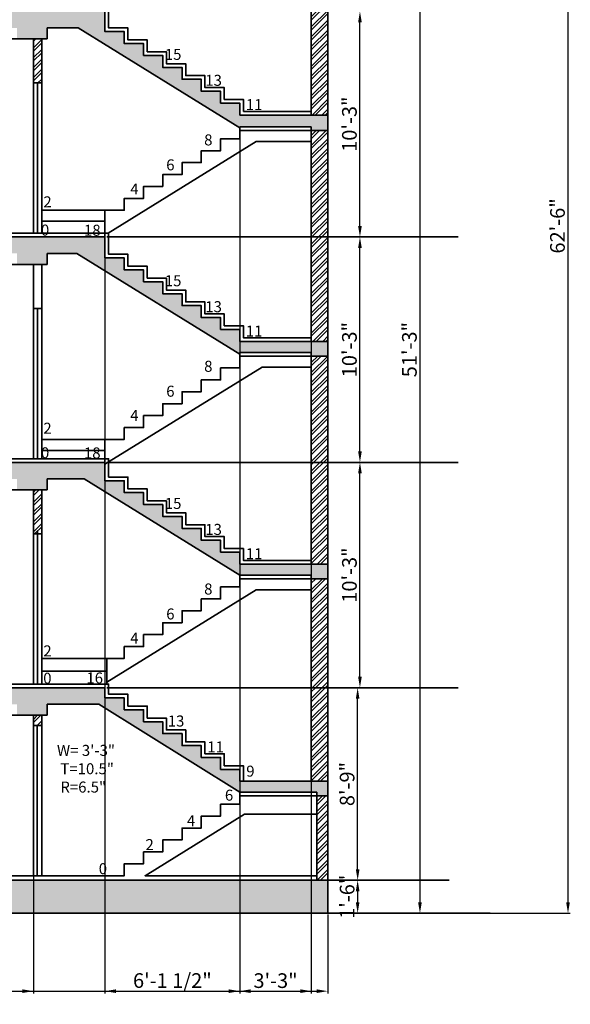
# Model space of a CAD drawing. Units: millimetres. Extents: x 1706 to 5913, y 156 to 1716.
# Tile 19 of 26: x 4807 to 5108, y 156 to 693. Entities that reach past the tile are written whole.
import ezdxf

# ---------------------------------------------------------------- set-up
doc = ezdxf.new("R2010")
doc.units = ezdxf.units.MM
for name, color, linetype, lineweight in [('A-ANNO-DIMS', 2, 'Continuous', 18), ('A-ANNO-TEXT', 7, 'Continuous', 18), ('A-SECT', 7, 'Continuous', 35), ('A-SECT-PATT', 8, 'Continuous', 13)]:
    doc.layers.add(name, color=color, linetype=linetype, lineweight=lineweight)
doc.styles.get("Standard").update_dxf_attribs({"font": 'arial.ttf'})
doc.dimstyles.new('ISO-25', dxfattribs={"dimtxt": 8, "dimasz": 6, "dimexe": 1.25, "dimexo": 0.625, "dimtad": 1, "dimdec": 0, "dimlunit": 3, "dimtxsty": 'Standard', "dimcen": 2.5, "dimadec": 0, "dimazin": 0, "dimtfac": 1, "dimtdec": 0, "dimtmove": 0, "dimatfit": 3, "dimfxl": 1, "dimarcsym": 0})
pattern_1 = [(45, (229.4607, 1496.8062), (-2.6940768, 2.6940768), []), (45, (231.2567, 1496.8062), (-2.6940768, 2.6940768), [])]
pattern_2 = [(50, (229.461, 1496.806), (14.574774, -1.275127), [1.524, -16.764]), (355, (229.46, 1496.806), (-2.819474, 15.284548), [1.2192, -13.411247]), (100.45144, (230.675, 1496.7), (11.7553, 14.00942), [1.2952, -14.24722]), (46.1842, (229.46, 1500.87), (21.68632, -3.363386), [2.286, -25.146]), (96.63556, (231.268, 1500.59), (18.99233, 19.79409), [1.9428, -21.37085]), (351.18415, (229.46, 1500.87), (18.99233, 19.79409), [1.8288, -20.11678]), (21, (231.493, 1499.854), (12.12915, -8.181216), [1.524, -16.764]), (326, (231.493, 1499.854), (4.94416, 14.735037), [1.2192, -13.4112]), (71.45144, (232.503, 1499.172), (17.073314, 6.55382), [1.2952, -14.247195]), (37.5, (229.4607, 1496.806), (0.247088, 6.764403), [0, -13.24864, 0, -13.6144, 0, -13.462]), (7.5, (229.461, 1496.806), (5.345573, 8.014446), [0, -7.76224, 0, -12.94384, 0, -5.1308]), (327.5, (224.9293, 1496.806), (10.8472476, -0.4582995), [0, -5.08, 0, -15.8496, 0, -21.0312]), (317.5, (222.897, 1496.806), (11.850335, 2.03412), [0, -6.604, 0, -10.52576, 0, -14.9352])]

# ---------------------------------------------------------------- blocks, each defined once
blk = doc.blocks.new('*D188')
at = {"layer": 'A-ANNO-DIMS', "color": 0, "lineweight": -2, "transparency": 16777216}
for p, q in [((4987.77, 328.75), (4992.93, 328.75)), ((4991.68, 229.75), (4991.68, 322.75)), ((4987.77, 223.75), (4992.93, 223.75))]:
    blk.add_line(p, q, dxfattribs=at)
at = {"layer": 'A-ANNO-DIMS', "color": 0, "transparency": 16777216}
for points in [[(4990.68, 322.75), (4992.68, 322.75), (4991.68, 328.75)], [(4990.68, 229.75), (4992.68, 229.75), (4991.68, 223.75)]]:
    blk.add_solid(points, dxfattribs=at)
at = {"layer": 'Defpoints', "color": 0, "transparency": 16777216}
for p in [(4987.15, 328.75), (4991.68, 328.75), (4987.15, 223.75)]:
    blk.add_point(p, dxfattribs=at)
at = {"layer": 'A-ANNO-DIMS', "color": 0, "transparency": 16777216, "insert": (4986.97, 276.25), "char_height": 8, "attachment_point": 5, "rotation": 90}
blk.add_mtext('8\'-9"', dxfattribs=at)
blk = doc.blocks.new('*D189')
at = {"layer": 'A-ANNO-DIMS', "color": 0, "lineweight": -2, "transparency": 16777216}
for p, q in [((4993.55, 451.75), (4994.18, 451.75)), ((4992.93, 334.75), (4992.93, 445.75)), ((4993.55, 328.75), (4994.18, 328.75))]:
    blk.add_line(p, q, dxfattribs=at)
at = {"layer": 'A-ANNO-DIMS', "color": 0, "transparency": 16777216}
for points in [[(4991.93, 445.75), (4993.93, 445.75), (4992.93, 451.75)], [(4991.93, 334.75), (4993.93, 334.75), (4992.93, 328.75)]]:
    blk.add_solid(points, dxfattribs=at)
at = {"layer": 'Defpoints', "color": 0, "transparency": 16777216}
for p in [(4992.93, 451.75), (4992.93, 451.75), (4992.93, 328.75)]:
    blk.add_point(p, dxfattribs=at)
at = {"layer": 'A-ANNO-DIMS', "color": 0, "transparency": 16777216, "insert": (4988.22, 390.25), "char_height": 8, "attachment_point": 5, "rotation": 90}
blk.add_mtext('10\'-3"', dxfattribs=at)
blk = doc.blocks.new('*D190')
at = {"layer": 'A-ANNO-DIMS', "color": 0, "lineweight": -2, "transparency": 16777216}
for p, q in [((4993.55, 574.75), (4994.18, 574.75)), ((4992.93, 457.75), (4992.93, 568.75)), ((4993.55, 451.75), (4994.18, 451.75))]:
    blk.add_line(p, q, dxfattribs=at)
at = {"layer": 'A-ANNO-DIMS', "color": 0, "transparency": 16777216}
for points in [[(4991.93, 568.75), (4993.93, 568.75), (4992.93, 574.75)], [(4991.93, 457.75), (4993.93, 457.75), (4992.93, 451.75)]]:
    blk.add_solid(points, dxfattribs=at)
at = {"layer": 'Defpoints', "color": 0, "transparency": 16777216}
for p in [(4992.93, 574.75), (4992.93, 574.75), (4992.93, 451.75)]:
    blk.add_point(p, dxfattribs=at)
at = {"layer": 'A-ANNO-DIMS', "color": 0, "transparency": 16777216, "insert": (4988.22, 513.25), "char_height": 8, "attachment_point": 5, "rotation": 90}
blk.add_mtext('10\'-3"', dxfattribs=at)
blk = doc.blocks.new('*D191')
at = {"layer": 'A-ANNO-DIMS', "color": 0, "lineweight": -2, "transparency": 16777216}
for p, q in [((4993.55, 697.75), (4991.68, 697.75)), ((4992.93, 580.75), (4992.93, 691.75)), ((4993.55, 574.75), (4991.68, 574.75))]:
    blk.add_line(p, q, dxfattribs=at)
at = {"layer": 'A-ANNO-DIMS', "color": 0, "transparency": 16777216}
for points in [[(4991.93, 691.75), (4993.93, 691.75), (4992.93, 697.75)], [(4991.93, 580.75), (4993.93, 580.75), (4992.93, 574.75)]]:
    blk.add_solid(points, dxfattribs=at)
at = {"layer": 'Defpoints', "color": 0, "transparency": 16777216}
for p in [(4992.93, 697.75), (4994.18, 697.75), (4994.18, 574.75)]:
    blk.add_point(p, dxfattribs=at)
at = {"layer": 'A-ANNO-DIMS', "color": 0, "transparency": 16777216, "insert": (4988.22, 636.25), "char_height": 8, "attachment_point": 5, "rotation": 90}
blk.add_mtext('10\'-3"', dxfattribs=at)
blk = doc.blocks.new('*D193')
at = {"layer": 'A-ANNO-DIMS', "color": 0, "lineweight": -2, "transparency": 16777216}
for p, q in [((5021.56, 820.75), (5026.89, 820.75)), ((5025.64, 814.75), (5025.64, 211.75)), ((5021.56, 205.75), (5026.89, 205.75))]:
    blk.add_line(p, q, dxfattribs=at)
at = {"layer": 'A-ANNO-DIMS', "color": 0, "transparency": 16777216}
for points in [[(5024.64, 814.75), (5026.64, 814.75), (5025.64, 820.75)], [(5024.64, 211.75), (5026.64, 211.75), (5025.64, 205.75)]]:
    blk.add_solid(points, dxfattribs=at)
at = {"layer": 'Defpoints', "color": 0, "transparency": 16777216}
for p in [(5020.94, 820.75), (5020.94, 205.75), (5025.64, 205.75)]:
    blk.add_point(p, dxfattribs=at)
at = {"layer": 'A-ANNO-DIMS', "color": 0, "transparency": 16777216, "insert": (5020.93, 513.25), "char_height": 8, "attachment_point": 5, "rotation": 90}
blk.add_mtext('51\'-3"', dxfattribs=at)
blk = doc.blocks.new('*D194')
at = {"layer": 'A-ANNO-DIMS', "color": 0, "lineweight": -2, "transparency": 16777216}
for p, q in [((4992.3, 223.75), (4992.93, 223.75)), ((4991.68, 217.75), (4991.68, 211.75)), ((4992.3, 205.75), (4992.93, 205.75))]:
    blk.add_line(p, q, dxfattribs=at)
at = {"layer": 'A-ANNO-DIMS', "color": 0, "transparency": 16777216}
for points in [[(4990.68, 217.75), (4992.68, 217.75), (4991.68, 223.75)], [(4990.68, 211.75), (4992.68, 211.75), (4991.68, 205.75)]]:
    blk.add_solid(points, dxfattribs=at)
at = {"layer": 'Defpoints', "color": 0, "transparency": 16777216}
for p in [(4991.68, 223.75), (4991.68, 205.75), (4991.68, 205.75)]:
    blk.add_point(p, dxfattribs=at)
at = {"layer": 'A-ANNO-DIMS', "color": 0, "transparency": 16777216, "insert": (4986.97, 214.75), "char_height": 8, "attachment_point": 5, "rotation": 90}
blk.add_mtext('1\'-6"', dxfattribs=at)
blk = doc.blocks.new('*D250')
at = {"layer": 'A-ANNO-DIMS', "color": 0, "lineweight": -2, "transparency": 16777216}
for p, q in [((4475.91, 205.12), (4475.91, 162)), ((4975.41, 205.12), (4975.41, 162)), ((4481.91, 163.25), (4969.41, 163.25))]:
    blk.add_line(p, q, dxfattribs=at)
at = {"layer": 'A-ANNO-DIMS', "color": 0, "transparency": 16777216}
for points in [[(4481.91, 164.25), (4481.91, 162.25), (4475.91, 163.25)], [(4969.41, 164.25), (4969.41, 162.25), (4975.41, 163.25)]]:
    blk.add_solid(points, dxfattribs=at)
at = {"layer": 'Defpoints', "color": 0, "transparency": 16777216}
for p in [(4475.91, 205.75), (4975.41, 205.75), (4975.41, 163.25)]:
    blk.add_point(p, dxfattribs=at)
at = {"layer": 'A-ANNO-DIMS', "color": 0, "transparency": 16777216, "insert": (4725.66, 168.01), "char_height": 8, "attachment_point": 5}
blk.add_mtext('41\'-7 1/2"', dxfattribs=at)
blk = doc.blocks.new('*D251')
at = {"layer": 'A-ANNO-DIMS', "color": 0, "lineweight": -2, "transparency": 16777216}
for p, q in [((4976.03, 955.75), (5107.63, 955.75)), ((5106.38, 211.75), (5106.38, 949.75)), ((4976.03, 205.75), (5107.63, 205.75))]:
    blk.add_line(p, q, dxfattribs=at)
at = {"layer": 'A-ANNO-DIMS', "color": 0, "transparency": 16777216}
for points in [[(5105.38, 949.75), (5107.38, 949.75), (5106.38, 955.75)], [(5105.38, 211.75), (5107.38, 211.75), (5106.38, 205.75)]]:
    blk.add_solid(points, dxfattribs=at)
at = {"layer": 'Defpoints', "color": 0, "transparency": 16777216}
for p in [(4975.41, 955.75), (5106.38, 955.75), (4975.41, 205.75)]:
    blk.add_point(p, dxfattribs=at)
at = {"layer": 'A-ANNO-DIMS', "color": 0, "transparency": 16777216, "insert": (5101.67, 580.75), "char_height": 8, "attachment_point": 5, "rotation": 90}
blk.add_mtext('62\'-6"', dxfattribs=at)
blk = doc.blocks.new('*D254')
at = {"layer": 'A-ANNO-DIMS', "color": 0, "lineweight": -2, "transparency": 16777216}
for p, q in [((4652.91, 330.12), (4652.91, 162)), ((4814.91, 225.62), (4814.91, 162)), ((4658.91, 163.25), (4808.91, 163.25))]:
    blk.add_line(p, q, dxfattribs=at)
at = {"layer": 'A-ANNO-DIMS', "color": 0, "transparency": 16777216}
for points in [[(4658.91, 164.25), (4658.91, 162.25), (4652.91, 163.25)], [(4808.91, 164.25), (4808.91, 162.25), (4814.91, 163.25)]]:
    blk.add_solid(points, dxfattribs=at)
at = {"layer": 'Defpoints', "color": 0, "transparency": 16777216}
for p in [(4652.91, 330.75), (4814.91, 226.25), (4814.91, 163.25)]:
    blk.add_point(p, dxfattribs=at)
at = {"layer": 'A-ANNO-DIMS', "color": 0, "transparency": 16777216, "insert": (4733.91, 167.96), "char_height": 8, "attachment_point": 5}
blk.add_mtext('13\'-6"', dxfattribs=at)
blk = doc.blocks.new('*D255')
at = {"layer": 'A-ANNO-DIMS', "color": 0, "lineweight": -2, "transparency": 16777216}
for p, q in [((4927.41, 634.12), (4927.41, 162)), ((4853.91, 588.62), (4853.91, 162)), ((4859.91, 163.25), (4921.41, 163.25))]:
    blk.add_line(p, q, dxfattribs=at)
at = {"layer": 'A-ANNO-DIMS', "color": 0, "transparency": 16777216}
for points in [[(4859.91, 164.25), (4859.91, 162.25), (4853.91, 163.25)], [(4921.41, 164.25), (4921.41, 162.25), (4927.41, 163.25)]]:
    blk.add_solid(points, dxfattribs=at)
at = {"layer": 'Defpoints', "color": 0, "transparency": 16777216}
for p in [(4927.41, 634.75), (4853.91, 589.25), (4927.41, 163.25)]:
    blk.add_point(p, dxfattribs=at)
at = {"layer": 'A-ANNO-DIMS', "color": 0, "transparency": 16777216, "insert": (4890.66, 168.01), "char_height": 8, "attachment_point": 5}
blk.add_mtext('6\'-1 1/2"', dxfattribs=at)
blk = doc.blocks.new('*D256')
at = {"layer": 'A-ANNO-DIMS', "color": 0, "lineweight": -2, "transparency": 16777216}
for p, q in [((4927.41, 634.12), (4927.41, 162)), ((4966.41, 634.12), (4966.41, 162)), ((4933.41, 163.25), (4960.41, 163.25))]:
    blk.add_line(p, q, dxfattribs=at)
at = {"layer": 'A-ANNO-DIMS', "color": 0, "transparency": 16777216}
for points in [[(4933.41, 164.25), (4933.41, 162.25), (4927.41, 163.25)], [(4960.41, 164.25), (4960.41, 162.25), (4966.41, 163.25)]]:
    blk.add_solid(points, dxfattribs=at)
at = {"layer": 'Defpoints', "color": 0, "transparency": 16777216}
for p in [(4927.41, 634.75), (4966.41, 634.75), (4966.41, 163.25)]:
    blk.add_point(p, dxfattribs=at)
at = {"layer": 'A-ANNO-DIMS', "color": 0, "transparency": 16777216, "insert": (4946.91, 167.96), "char_height": 8, "attachment_point": 5}
blk.add_mtext('3\'-3"', dxfattribs=at)

msp = doc.modelspace()

# ---------------------------------------------------------------- hatches: boundary and pattern name
at = {"layer": 'A-SECT-PATT'}
h = msp.add_hatch(dxfattribs=at)
h.set_pattern_fill('ANSI32', color=256, scale=0.4)
h.set_pattern_definition(pattern_1)
h.paths.add_polyline_path([(4975.41, 755.75), (4966.41, 755.75), (4966.41, 641.25), (4975.41, 641.25)])
h = msp.add_hatch(dxfattribs=at)
h.set_pattern_fill('AR-CONC', color=256, scale=0.08)
h.set_pattern_definition(pattern_2)
h.paths.add_polyline_path([(4853.91, 697.75), (4475.91, 697.75), (4475.91, 682.75), (4484.91, 682.75), (4484.91, 688.75), (4805.91, 688.75), (4805.91, 682.75), (4822.41, 682.75), (4822.41, 688.75), (4839.28, 688.75), (4927.41, 634.19), (4927.41, 634.75), (4966.41, 634.75), (4966.41, 632.75), (4975.41, 632.75), (4975.41, 641.25), (4927.41, 641.25), (4927.41, 647.75), (4916.91, 647.75), (4916.91, 654.25), (4906.41, 654.25), (4906.41, 660.75), (4895.91, 660.75), (4895.91, 667.25), (4885.41, 667.25), (4885.41, 673.75), (4874.91, 673.75), (4874.91, 680.25), (4864.41, 680.25), (4864.41, 686.75), (4853.91, 686.75)])
h = msp.add_hatch(dxfattribs=at)
h.set_pattern_fill('ANSI32', color=256, scale=0.4)
h.set_pattern_definition(pattern_1)
h.paths.add_polyline_path([(4819.41, 682.75), (4814.91, 682.75), (4814.91, 658.75), (4819.41, 658.75)])
h = msp.add_hatch(dxfattribs=at)
h.set_pattern_fill('ANSI32', color=256, scale=0.4)
h.set_pattern_definition(pattern_1)
h.paths.add_polyline_path([(4975.41, 632.75), (4966.41, 632.75), (4966.41, 517.75), (4975.41, 517.75)])
h = msp.add_hatch(dxfattribs=at)
h.set_pattern_fill('AR-CONC', color=256, scale=0.08)
h.set_pattern_definition(pattern_2)
h.paths.add_polyline_path([(4853.91, 569.75), (4853.91, 574.75), (4475.91, 574.75), (4475.91, 559.75), (4484.91, 559.75), (4484.91, 565.75), (4805.91, 565.75), (4805.91, 559.75), (4822.41, 559.75), (4822.41, 565.75), (4838.47, 565.75), (4927.41, 510.69), (4927.41, 511.75), (4966.41, 511.75), (4966.41, 509.75), (4975.41, 509.75), (4975.41, 517.75), (4927.41, 517.75), (4927.41, 524.25), (4916.91, 524.25), (4916.91, 530.75), (4906.41, 530.75), (4906.41, 537.25), (4895.91, 537.25), (4895.91, 543.75), (4885.41, 543.75), (4885.41, 550.25), (4874.91, 550.25), (4874.91, 556.75), (4864.41, 556.75), (4864.41, 563.25), (4853.91, 563.25)])
h = msp.add_hatch(dxfattribs=at)
h.set_pattern_fill('ANSI32', color=256, scale=0.4)
h.set_pattern_definition(pattern_1)
h.paths.add_polyline_path([(4975.41, 509.75), (4966.41, 509.75), (4966.41, 396.25), (4975.41, 396.25)])
h = msp.add_hatch(dxfattribs=at)
h.set_pattern_fill('AR-CONC', color=256, scale=0.08)
h.set_pattern_definition(pattern_2)
h.paths.add_polyline_path([(4853.91, 451.75), (4475.91, 451.75), (4475.91, 436.75), (4484.91, 436.75), (4484.91, 442.75), (4805.91, 442.75), (4805.91, 436.75), (4822.41, 436.75), (4822.41, 442.75), (4842.6, 442.75), (4927.41, 390.25), (4966.41, 390.25), (4966.41, 388.25), (4975.41, 388.25), (4975.41, 396.25), (4927.41, 396.25), (4927.41, 402.75), (4916.91, 402.75), (4916.91, 409.25), (4906.41, 409.25), (4906.41, 415.75), (4895.91, 415.75), (4895.91, 422.25), (4885.41, 422.25), (4885.41, 428.75), (4874.91, 428.75), (4874.91, 435.25), (4864.41, 435.25), (4864.41, 441.75), (4853.91, 441.75)])
h = msp.add_hatch(dxfattribs=at)
h.set_pattern_fill('ANSI32', color=256, scale=0.4)
h.set_pattern_definition(pattern_1)
h.paths.add_polyline_path([(4819.41, 436.75), (4814.91, 436.75), (4814.91, 412.75), (4819.41, 412.75)])
h = msp.add_hatch(dxfattribs=at)
h.set_pattern_fill('ANSI32', color=256, scale=0.4)
h.set_pattern_definition(pattern_1)
h.paths.add_polyline_path([(4975.41, 388.25), (4966.41, 388.25), (4966.41, 328.75), (4975.41, 328.75)])
h = msp.add_hatch(dxfattribs=at)
h.set_pattern_fill('AR-CONC', color=256, scale=0.08)
h.set_pattern_definition(pattern_2)
h.paths.add_polyline_path([(4864.41, 323.25), (4853.91, 323.25), (4853.91, 328.75), (4475.91, 328.75), (4475.91, 319.75), (4805.91, 319.75), (4805.91, 313.75), (4814.91, 313.75), (4822.41, 313.75), (4822.41, 319.75), (4850.55, 319.75), (4927.41, 271.75), (4969.41, 271.75), (4969.41, 269.75), (4975.41, 269.75), (4975.41, 277.75), (4927.41, 277.75), (4927.41, 284.25), (4916.91, 284.25), (4916.91, 290.75), (4906.41, 290.75), (4906.41, 297.25), (4895.91, 297.25), (4895.91, 303.75), (4885.41, 303.75), (4885.41, 310.25), (4874.91, 310.25), (4874.91, 316.75), (4864.41, 316.75)])
h = msp.add_hatch(dxfattribs=at)
h.set_pattern_fill('ANSI32', color=256, scale=0.4)
h.set_pattern_definition(pattern_1)
h.paths.add_polyline_path([(4975.41, 328.75), (4966.41, 328.75), (4966.41, 277.75), (4975.41, 277.75)])
h = msp.add_hatch(dxfattribs=at)
h.set_pattern_fill('ANSI32', color=256, scale=0.4)
h.set_pattern_definition(pattern_1)
h.paths.add_polyline_path([(4819.41, 313.75), (4814.91, 313.75), (4814.91, 308.19), (4819.41, 308.19)])
h = msp.add_hatch(dxfattribs=at)
h.set_pattern_fill('ANSI32', color=256, scale=0.4)
h.set_pattern_definition(pattern_1)
h.paths.add_polyline_path([(4975.41, 269.75), (4969.41, 269.75), (4969.41, 223.75), (4975.41, 223.75)])
h = msp.add_hatch(dxfattribs=at)
h.set_pattern_fill('AR-CONC', color=256, scale=0.08)
h.set_pattern_definition(pattern_2)
h.paths.add_polyline_path([(4975.41, 223.75), (4475.91, 223.75), (4475.91, 205.75), (4975.41, 205.75)])

# ---------------------------------------------------------------- linework, layer by layer
at = {"layer": 'A-SECT'}
for p, q in [((4975.41, 955.75), (4975.41, 205.75)), ((4966.41, 757.75), (4966.41, 641.25)), ((4822.41, 688.75), (4839.28, 688.75)), ((4822.41, 682.75), (4822.41, 688.75)), ((4927.41, 634.19), (4839.28, 688.75)), ((4657.41, 682.75), (4822.41, 682.75)), ((4814.91, 682.75), (4814.91, 576.75)), ((4819.41, 682.75), (4819.41, 576.75)), ((4814.91, 658.75), (4819.41, 658.75)), ((4817.16, 658.75), (4817.16, 576.75)), ((4927.41, 641.25), (4975.41, 641.25)), ((4929.41, 643.25), (4966.41, 643.25)), ((4927.41, 634.75), (4966.41, 634.75)), ((4966.41, 634.75), (4966.41, 517.75)), ((4927.41, 632.75), (4966.41, 632.75)), ((4966.41, 632.75), (4975.41, 632.75)), ((4936.38, 626.75), (4855.61, 576.75)), ((4936.38, 626.75), (4966.41, 626.75)), ((4853.91, 589.25), (4819.41, 589.25)), ((4853.91, 589.25), (4853.91, 574.75)), ((4853.91, 583.25), (4819.41, 583.25)), ((4475.91, 574.75), (4853.91, 574.75)), ((4854.91, 574.75), (5046.51, 574.75)), ((4822.41, 559.75), (4822.41, 565.75)), ((4822.41, 565.75), (4838.47, 565.75)), ((4927.41, 510.69), (4838.47, 565.75)), ((4657.41, 559.75), (4822.41, 559.75)), ((4814.91, 559.75), (4814.91, 453.75)), ((4819.41, 559.75), (4819.41, 453.75)), ((4814.91, 535.75), (4819.41, 535.75)), ((4817.16, 535.75), (4817.16, 453.75)), ((4927.41, 511.75), (4927.41, 509.75)), ((4927.41, 511.75), (4966.41, 511.75)), ((4966.41, 511.75), (4966.41, 396.25)), ((4927.41, 509.75), (4966.41, 509.75)), ((4966.41, 509.75), (4975.41, 509.75)), ((4939.61, 503.75), (4853.91, 450.69)), ((4939.61, 503.75), (4966.41, 503.75)), ((4853.91, 464.25), (4819.41, 464.25)), ((4853.91, 458.25), (4819.41, 458.25)), ((4475.91, 451.75), (4853.91, 451.75)), ((4854.91, 451.75), (5046.51, 451.75)), ((4822.41, 442.75), (4842.6, 442.75)), ((4822.41, 436.75), (4822.41, 442.75)), ((4927.41, 390.25), (4842.6, 442.75)), ((4657.41, 436.75), (4822.41, 436.75)), ((4814.91, 436.75), (4814.91, 330.75)), ((4819.41, 436.75), (4819.41, 330.75)), ((4817.16, 414.33), (4817.16, 330.75)), ((4814.91, 412.75), (4819.41, 412.75)), ((4927.41, 390.25), (4966.41, 390.25)), ((4927.41, 390.25), (4927.41, 383.75)), ((4927.41, 388.25), (4966.41, 388.25)), ((4966.41, 390.25), (4966.41, 277.75)), ((4966.41, 388.25), (4975.41, 388.25)), ((4936.38, 382.25), (4854.91, 331.81)), ((4936.38, 382.25), (4966.41, 382.25)), ((4854.91, 344.75), (4819.41, 344.75)), ((4854.91, 330.75), (4854.91, 344.75)), ((4854.91, 337.75), (4819.41, 337.75)), ((4475.91, 328.75), (4853.91, 328.75)), ((4854.91, 328.75), (5046.51, 328.75)), ((4822.41, 319.75), (4822.41, 313.75)), ((4822.41, 319.75), (4850.55, 319.75)), ((4927.41, 271.75), (4850.55, 319.75)), ((4814.91, 313.75), (4790.91, 313.75)), ((4808.91, 313.75), (4822.41, 313.75)), ((4814.91, 313.75), (4814.91, 226.25)), ((4819.41, 313.75), (4819.41, 226.25)), ((4814.91, 308.19), (4819.41, 308.19)), ((4817, 308.19), (4817, 226.25)), ((4927.41, 277.75), (4975.41, 277.75)), ((4927.41, 271.75), (4969.41, 271.75)), ((4927.41, 269.75), (4966.41, 269.75)), ((4966.41, 269.75), (4975.41, 269.75)), ((4969.41, 271.75), (4969.41, 223.75)), ((4475.91, 223.75), (4975.41, 223.75)), ((4975.41, 223.75), (5041.62, 223.75)), ((4475.91, 205.75), (4975.41, 205.75)), ((4975.41, 205.75), (5063.88, 205.75))]:
    msp.add_line(p, q, dxfattribs=at)
for points in [[(4929.41, 643.25), (4929.41, 649.75), (4918.91, 649.75), (4918.91, 656.25), (4908.41, 656.25), (4908.41, 662.75), (4897.91, 662.75), (4897.91, 669.25), (4887.41, 669.25), (4887.41, 675.75), (4876.91, 675.75), (4876.91, 682.25), (4866.41, 682.25), (4866.41, 688.75), (4855.91, 688.75), (4855.91, 699.75), (4475.91, 699.75)], [(4927.41, 641.25), (4927.41, 647.75), (4916.91, 647.75), (4916.91, 654.25), (4906.41, 654.25), (4906.41, 660.75), (4895.91, 660.75), (4895.91, 667.25), (4885.41, 667.25), (4885.41, 673.75), (4874.91, 673.75), (4874.91, 680.25), (4864.41, 680.25), (4864.41, 686.75), (4853.91, 686.75), (4853.91, 697.75)], [(4927.41, 634.75), (4927.41, 628.25), (4916.91, 628.25), (4916.91, 621.75), (4906.41, 621.75), (4906.41, 615.25), (4895.91, 615.25), (4895.91, 608.75), (4885.41, 608.75), (4885.41, 602.25), (4874.91, 602.25), (4874.91, 595.75), (4864.41, 595.75), (4864.41, 589.25), (4853.91, 589.25)], [(4966.41, 519.75), (4929.41, 519.75), (4929.41, 526.25), (4918.91, 526.25), (4918.91, 532.75), (4908.41, 532.75), (4908.41, 539.25), (4897.91, 539.25), (4897.91, 545.75), (4887.41, 545.75), (4887.41, 552.25), (4876.91, 552.25), (4876.91, 558.75), (4866.41, 558.75), (4866.41, 565.25), (4855.91, 565.25), (4855.91, 569.75), (4855.91, 576.75), (4475.91, 576.75)], [(4975.41, 517.75), (4927.41, 517.75), (4927.41, 524.25), (4916.91, 524.25), (4916.91, 530.75), (4906.41, 530.75), (4906.41, 537.25), (4895.91, 537.25), (4895.91, 543.75), (4885.41, 543.75), (4885.41, 550.25), (4874.91, 550.25), (4874.91, 556.75), (4864.41, 556.75), (4864.41, 563.25), (4853.91, 563.25), (4853.91, 569.75), (4853.91, 574.75)], [(4927.41, 509.75), (4927.41, 503.25), (4916.91, 503.25), (4916.91, 496.75), (4906.41, 496.75), (4906.41, 490.25), (4895.91, 490.25), (4895.91, 483.75), (4885.41, 483.75), (4885.41, 477.25), (4874.91, 477.25), (4874.91, 470.75), (4864.41, 470.75), (4864.41, 464.25), (4853.91, 464.25), (4853.91, 451.75)], [(4966.41, 398.25), (4929.41, 398.25), (4929.41, 404.75), (4918.91, 404.75), (4918.91, 411.25), (4908.41, 411.25), (4908.41, 417.75), (4897.91, 417.75), (4897.91, 424.25), (4887.41, 424.25), (4887.41, 430.75), (4876.91, 430.75), (4876.91, 437.25), (4866.41, 437.25), (4866.41, 443.75), (4855.91, 443.75), (4855.91, 453.75), (4475.91, 453.75)], [(4975.41, 396.25), (4927.41, 396.25), (4927.41, 402.75), (4916.91, 402.75), (4916.91, 409.25), (4906.41, 409.25), (4906.41, 415.75), (4895.91, 415.75), (4895.91, 422.25), (4885.41, 422.25), (4885.41, 428.75), (4874.91, 428.75), (4874.91, 435.25), (4864.41, 435.25), (4864.41, 441.75), (4853.91, 441.75), (4853.91, 451.75)], [(4927.41, 383.75), (4916.91, 383.75), (4916.91, 377.25), (4906.41, 377.25), (4906.41, 370.75), (4895.91, 370.75), (4895.91, 364.25), (4885.41, 364.25), (4885.41, 357.75), (4874.91, 357.75), (4874.91, 351.25), (4864.41, 351.25), (4864.41, 344.75), (4854.91, 344.75)], [(4929.41, 277.75), (4929.41, 286.25), (4918.91, 286.25), (4918.91, 292.75), (4908.41, 292.75), (4908.41, 299.25), (4897.91, 299.25), (4897.91, 305.75), (4887.41, 305.75), (4887.41, 312.25), (4876.91, 312.25), (4876.91, 318.75), (4866.41, 318.75), (4866.41, 325.25), (4855.91, 325.25), (4855.91, 330.75), (4475.91, 330.75)], [(4927.41, 277.75), (4927.41, 284.25), (4916.91, 284.25), (4916.91, 290.75), (4906.41, 290.75), (4906.41, 297.25), (4895.91, 297.25), (4895.91, 303.75), (4885.41, 303.75), (4885.41, 310.25), (4874.91, 310.25), (4874.91, 316.75), (4864.41, 316.75), (4864.41, 323.25), (4853.91, 323.25), (4853.91, 328.75)], [(4927.41, 271.75), (4927.41, 265.25), (4916.91, 265.25), (4916.91, 258.75), (4906.41, 258.75), (4906.41, 252.25), (4895.91, 252.25), (4895.91, 245.75), (4885.41, 245.75), (4885.41, 239.25), (4874.91, 239.25), (4874.91, 232.75), (4864.41, 232.75), (4864.41, 226.25), (4484.91, 226.25)], [(4969.41, 226.25), (4875.8, 226.25), (4929.92, 259.75), (4969.41, 259.75)]]:
    msp.add_lwpolyline(points, dxfattribs=at)

# ---------------------------------------------------------------- texts
at = {"layer": 'A-ANNO-TEXT', "char_height": 6, "attachment_point": 1}
for s, width, insert in [(' 15', 13.3033, (4884.68, 677.33)), (' 13', 13.3033, (4906.74, 663.17)), (' 11', 13.3033, (4928.86, 649.89)), (' 8', 13.3033, (4906.15, 630.66)), (' 6', 13.3033, (4885.46, 617.05)), (' 4', 13.3033, (4865.85, 603.88)), (' 2', 13.3033, (4818.45, 596.87)), (' 0', 13.3033, (4817.15, 581.48)), (' 18', 13.3033, (4840.6, 581.38)), (' 15', 13.3033, (4884.68, 553.83)), (' 13', 13.3033, (4906.74, 539.67)), (' 11', 13.3033, (4928.86, 526.39)), (' 8', 13.3033, (4906.15, 507.16)), (' 6', 13.3033, (4885.46, 493.55)), (' 4', 13.3033, (4865.85, 480.38)), (' 2', 13.3033, (4818.45, 473.37)), (' 0', 13.3033, (4817.15, 459.98)), (' 18', 13.3033, (4840.6, 459.88)), (' 15', 13.3033, (4884.68, 432.33)), (' 13', 13.3033, (4906.74, 418.17)), (' 11', 13.3033, (4928.86, 404.89)), (' 8', 13.3033, (4906.15, 385.66)), (' 6', 13.3033, (4885.46, 372.05)), (' 4', 13.3033, (4865.85, 358.88)), (' 2', 13.3033, (4818.45, 351.87)), (' 0', 13.3033, (4818.4, 336.98)), (' 16', 13.3033, (4841.93, 337.12)), (' 13', 13.3033, (4886.29, 313.64)), ('   W= 3\'-3"\\P    T=10.5"\\P    R=6.5"', 67.9131, (4822.22, 297.61)), (' 11', 13.3033, (4907.87, 299.51)), (' 9', 13.3033, (4929.1, 286.28)), (' 6', 13.3033, (4917.46, 273.17)), (' 4', 13.3033, (4896.74, 259.25)), (' 2', 13.3033, (4874.17, 246.22)), (' 0', 13.3033, (4848.66, 233.06))]:
    msp.add_mtext_dynamic_manual_height_columns(s, width=width, gutter_width=12.5, heights=[0], dxfattribs=dict(at, insert=insert))

# ---------------------------------------------------------------- dimensions: what is measured, and where the dimension line sits
at = {"layer": 'A-ANNO-DIMS'}
for base, p1, p2, override, picture, middle in [((5106.38, 955.75), (4975.41, 205.75), (4975.41, 955.75), {"dimdec": 1, "dimlfac": 1, "dimrnd": 0, "dimzin": 1, "dimdsep": 46, "dimlunit": 4, "dimfrac": 2}, '*D251', (5101.67, 580.75)), ((5025.64, 205.75), (5020.94, 820.75), (5020.94, 205.75), {"dimclrd": 0, "dimclre": 0, "dimclrt": 0}, '*D193', (5020.93, 513.25)), ((4992.93, 697.75), (4994.18, 574.75), (4994.18, 697.75), {"dimclrd": 0, "dimclre": 0, "dimclrt": 0}, '*D191', (4988.22, 636.25)), ((4992.93, 574.75), (4992.93, 451.75), (4992.93, 574.75), {"dimclrd": 0, "dimclre": 0, "dimclrt": 0}, '*D190', (4988.22, 513.25)), ((4992.93, 451.75), (4992.93, 328.75), (4992.93, 451.75), {"dimclrd": 0, "dimclre": 0, "dimclrt": 0}, '*D189', (4988.22, 390.25)), ((4991.68, 328.75), (4987.15, 223.75), (4987.15, 328.75), {"dimclrd": 0, "dimclre": 0, "dimclrt": 0}, '*D188', (4986.97, 276.25))]:
    dim = msp.add_linear_dim(base=base, p1=p1, p2=p2, angle=90, dimstyle='ISO-25', override=override, dxfattribs=at)
    dim.commit()
    dim.dimension.update_dxf_attribs({"geometry": picture, "text_midpoint": middle})
for base, p1, p2, picture, middle in [((4927.41, 163.25), (4853.91, 589.25), (4927.41, 634.75), '*D255', (4890.66, 168.01)), ((4966.41, 163.25), (4927.41, 634.75), (4966.41, 634.75), '*D256', (4946.91, 167.96)), ((4814.91, 163.25), (4652.91, 330.75), (4814.91, 226.25), '*D254', (4733.91, 167.96)), ((4975.41, 163.25), (4475.91, 205.75), (4975.41, 205.75), '*D250', (4725.66, 168.01))]:
    dim = msp.add_linear_dim(base=base, p1=p1, p2=p2, dimstyle='ISO-25', override={"dimdec": 1, "dimlfac": 1, "dimrnd": 0, "dimzin": 1, "dimdsep": 46, "dimlunit": 4, "dimfrac": 2}, dxfattribs=at)
    dim.commit()
    dim.dimension.update_dxf_attribs({"geometry": picture, "text_midpoint": middle})
dim = msp.add_linear_dim(base=(4991.68, 205.75), p1=(4991.68, 223.75), p2=(4991.68, 205.75), angle=90, dimstyle='ISO-25', override={"dimclrd": 0, "dimclre": 0, "dimclrt": 0}, dxfattribs=at)
dim.commit()
dim.dimension.update_dxf_attribs({"geometry": '*D194', "text_midpoint": (4991.68, 214.75), "dimtype": 160})

doc.saveas('drawing.dxf')
